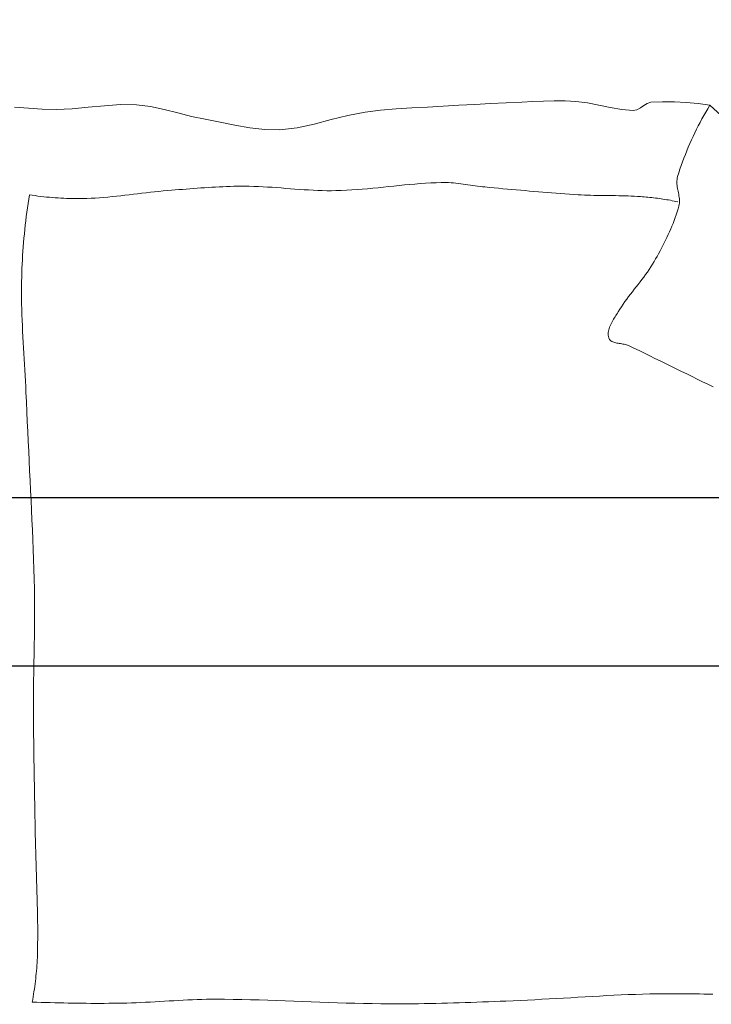
# Model space of a CAD drawing. Units: inches. Extents: x 1484 to 2008, y 1843 to 2590.
# Tile 5 of 21: x 1811 to 1853, y 1981 to 2039. Entities that reach past the tile are written whole.
import ezdxf

# ---------------------------------------------------------------- set-up
doc = ezdxf.new("R2010")
doc.units = ezdxf.units.IN
doc.layers.add('A-ANNO-DIMS', color=2, linetype='Continuous', lineweight=18)
doc.layers.add('A-FURN', color=8, linetype='Continuous', lineweight=18)
doc.styles.get("Standard").update_dxf_attribs({"font": 'arial.ttf'})
doc.dimstyles.new('ISO-25', dxfattribs={"dimtxt": 7, "dimasz": 2.5, "dimexe": 1.25, "dimexo": 0.625, "dimtad": 1, "dimdec": 0, "dimlunit": 3, "dimtxsty": 'Standard', "dimcen": 2.5, "dimadec": 0, "dimazin": 0, "dimtfac": 1, "dimtdec": 0, "dimtmove": 0, "dimatfit": 3, "dimfxl": 1, "dimarcsym": 0})

# ---------------------------------------------------------------- blocks, each defined once
blk = doc.blocks.new('BED-DOUBLE')
for p, q in [((1.063, 49.042), (0.265, 48.148)), ((0.265, 48.148), (0.164, 47.454)), ((0.265, 48.148), (0.464, 48.028)), ((0.464, 48.028), (0.665, 47.91)), ((0.665, 47.91), (0.867, 47.795)), ((16.669, 47.725), (16.821, 48.04)), ((16.821, 48.04), (16.973, 48.355)), ((53.003, 47.799), (53.009, 48.067)), ((53.009, 48.067), (53.016, 48.334)), ((0.164, 47.454), (0.095, 46.755)), ((0.867, 47.795), (1.07, 47.682)), ((1.07, 47.682), (1.275, 47.572)), ((1.275, 47.572), (1.482, 47.465)), ((1.482, 47.465), (1.69, 47.36)), ((1.69, 47.36), (1.899, 47.258)), ((16.362, 47.096), (16.516, 47.41)), ((16.516, 47.41), (16.669, 47.725)), ((52.992, 47.265), (52.997, 47.532)), ((52.997, 47.532), (53.003, 47.799)), ((0.095, 46.755), (0.059, 46.053)), ((1.899, 47.258), (2.11, 47.158)), ((2.11, 47.158), (2.322, 47.061)), ((2.322, 47.061), (2.535, 46.966)), ((2.535, 46.966), (2.749, 46.875)), ((2.749, 46.875), (2.964, 46.786)), ((2.964, 46.786), (3.18, 46.699)), ((16.053, 46.467), (16.208, 46.781)), ((16.208, 46.781), (16.362, 47.096)), ((52.983, 46.731), (52.987, 46.998)), ((52.987, 46.998), (52.992, 47.265)), ((3.18, 46.699), (3.398, 46.616)), ((3.398, 46.616), (3.616, 46.535)), ((3.616, 46.535), (3.835, 46.457)), ((3.835, 46.457), (4.055, 46.382)), ((4.055, 46.382), (4.276, 46.31)), ((4.276, 46.31), (4.498, 46.24)), ((4.498, 46.24), (4.581, 46.219)), ((4.581, 46.219), (4.666, 46.205)), ((4.666, 46.205), (4.752, 46.198)), ((4.752, 46.198), (4.839, 46.197)), ((4.839, 46.197), (4.926, 46.202)), ((4.926, 46.202), (5.014, 46.211)), ((5.014, 46.211), (5.102, 46.223)), ((5.102, 46.223), (5.191, 46.238)), ((5.191, 46.238), (5.279, 46.254)), ((5.279, 46.254), (5.368, 46.272)), ((5.368, 46.272), (5.457, 46.29)), ((5.457, 46.29), (5.546, 46.307)), ((5.546, 46.307), (5.635, 46.322)), ((5.635, 46.322), (5.723, 46.335)), ((5.723, 46.335), (5.811, 46.345)), ((5.811, 46.345), (5.899, 46.351)), ((5.899, 46.351), (5.986, 46.352)), ((5.989, 46.252), (5.966, 46.142)), ((5.986, 46.352), (6.072, 46.347)), ((6.072, 46.347), (6.158, 46.335)), ((6.158, 46.335), (6.242, 46.316)), ((6.242, 46.316), (6.416, 46.266)), ((6.416, 46.266), (6.588, 46.213)), ((6.588, 46.213), (6.76, 46.157)), ((6.76, 46.157), (6.931, 46.097)), ((15.898, 46.154), (16.053, 46.467)), ((52.978, 45.93), (52.979, 46.197)), ((52.979, 46.197), (52.981, 46.464)), ((52.981, 46.464), (52.983, 46.731)), ((0.059, 46.053), (0.056, 45.35)), ((5.864, 45.592), (5.846, 45.481)), ((5.883, 45.702), (5.864, 45.592)), ((5.903, 45.812), (5.883, 45.702)), ((5.923, 45.923), (5.903, 45.812)), ((5.944, 46.032), (5.923, 45.923)), ((5.966, 46.142), (5.944, 46.032)), ((6.931, 46.097), (7.1, 46.035)), ((7.1, 46.035), (7.269, 45.97)), ((7.269, 45.97), (7.437, 45.903)), ((7.437, 45.903), (7.604, 45.833)), ((7.604, 45.833), (7.77, 45.76)), ((7.77, 45.76), (7.935, 45.686)), ((7.935, 45.686), (8.1, 45.609)), ((8.1, 45.609), (8.263, 45.53)), ((15.589, 45.526), (15.743, 45.84)), ((15.743, 45.84), (15.898, 46.154)), ((52.978, 45.663), (52.978, 45.93)), ((52.98, 45.396), (52.978, 45.663)), ((0.056, 45.35), (0.087, 44.65)), ((5.782, 45.038), (5.767, 44.927)), ((5.797, 45.149), (5.782, 45.038)), ((5.812, 45.26), (5.797, 45.149)), ((5.829, 45.371), (5.812, 45.26)), ((5.846, 45.481), (5.829, 45.371)), ((8.263, 45.53), (8.426, 45.45)), ((8.426, 45.45), (8.587, 45.368)), ((8.587, 45.368), (8.748, 45.284)), ((8.748, 45.284), (8.908, 45.199)), ((8.908, 45.199), (9.068, 45.113)), ((9.068, 45.113), (9.226, 45.025)), ((9.226, 45.025), (9.384, 44.936)), ((15.28, 44.897), (15.434, 45.212)), ((15.434, 45.212), (15.589, 45.526)), ((52.983, 45.129), (52.98, 45.396)), ((52.987, 44.862), (52.983, 45.129)), ((0.087, 44.65), (0.148, 44.431)), ((0.148, 44.431), (0.271, 44.228)), ((5.718, 44.482), (5.707, 44.371)), ((5.729, 44.593), (5.718, 44.482)), ((5.741, 44.705), (5.729, 44.593)), ((5.754, 44.816), (5.741, 44.705)), ((5.767, 44.927), (5.754, 44.816)), ((9.384, 44.936), (9.541, 44.847)), ((9.541, 44.847), (9.699, 44.754)), ((9.699, 44.754), (9.854, 44.656)), ((9.854, 44.656), (10.007, 44.555)), ((10.007, 44.555), (10.158, 44.451)), ((10.158, 44.451), (10.307, 44.345)), ((14.974, 44.268), (15.127, 44.583)), ((15.127, 44.583), (15.28, 44.897)), ((52.993, 44.595), (52.987, 44.862)), ((53.005, 44.167), (52.993, 44.595)), ((0.271, 44.228), (0.412, 44.029)), ((0.412, 44.029), (0.528, 43.826)), ((0.528, 43.826), (0.574, 43.607)), ((5.668, 43.852), (5.658, 43.667)), ((5.68, 44.036), (5.668, 43.852)), ((5.688, 44.148), (5.68, 44.036)), ((5.697, 44.259), (5.688, 44.148)), ((5.707, 44.371), (5.697, 44.259)), ((10.307, 44.345), (10.455, 44.236)), ((10.455, 44.236), (10.602, 44.125)), ((10.602, 44.125), (10.748, 44.013)), ((10.748, 44.013), (10.893, 43.9)), ((10.893, 43.9), (11.037, 43.786)), ((14.671, 43.637), (14.822, 43.953)), ((14.822, 43.953), (14.974, 44.268)), ((53.02, 43.74), (53.005, 44.167)), ((0.574, 43.607), (0.52, 42.921)), ((5.643, 43.298), (5.637, 43.113)), ((5.65, 43.483), (5.643, 43.298)), ((5.658, 43.667), (5.65, 43.483)), ((11.037, 43.786), (11.182, 43.672)), ((11.182, 43.672), (11.327, 43.559)), ((11.327, 43.559), (11.472, 43.446)), ((11.472, 43.446), (11.619, 43.334)), ((11.619, 43.334), (11.766, 43.224)), ((14.476, 43.199), (14.497, 43.262)), ((14.497, 43.262), (14.522, 43.32)), ((14.522, 43.32), (14.671, 43.637)), ((53.036, 43.313), (53.02, 43.74)), ((53.055, 42.886), (53.036, 43.313)), ((0.52, 42.921), (0.401, 42.241)), ((5.629, 42.744), (5.626, 42.559)), ((5.633, 42.929), (5.629, 42.744)), ((5.637, 43.113), (5.633, 42.929)), ((11.766, 43.224), (11.914, 43.116)), ((11.914, 43.116), (12.064, 43.01)), ((12.064, 43.01), (12.216, 42.907)), ((12.216, 42.907), (12.37, 42.807)), ((12.37, 42.807), (12.526, 42.712)), ((12.526, 42.712), (12.597, 42.669)), ((12.597, 42.669), (12.668, 42.624)), ((14.372, 42.642), (14.385, 42.711)), ((14.385, 42.711), (14.396, 42.782)), ((14.396, 42.782), (14.407, 42.853)), ((14.407, 42.853), (14.418, 42.925)), ((14.418, 42.925), (14.43, 42.996)), ((14.43, 42.996), (14.443, 43.066)), ((14.443, 43.066), (14.459, 43.134)), ((14.459, 43.134), (14.476, 43.199)), ((53.075, 42.458), (53.055, 42.886)), ((0.401, 42.241), (0.255, 41.563)), ((5.621, 42.189), (5.619, 42.005)), ((5.624, 42.374), (5.621, 42.189)), ((5.626, 42.559), (5.624, 42.374)), ((12.668, 42.624), (12.741, 42.578)), ((12.741, 42.578), (12.814, 42.532)), ((12.814, 42.532), (12.889, 42.485)), ((12.889, 42.485), (12.964, 42.439)), ((12.964, 42.439), (13.04, 42.394)), ((13.04, 42.394), (13.116, 42.35)), ((13.116, 42.35), (13.194, 42.309)), ((13.194, 42.309), (13.271, 42.27)), ((13.271, 42.27), (13.349, 42.234)), ((13.349, 42.234), (13.427, 42.203)), ((13.427, 42.203), (13.506, 42.176)), ((13.506, 42.176), (13.585, 42.153)), ((13.585, 42.153), (13.663, 42.137)), ((13.663, 42.137), (13.742, 42.126)), ((13.742, 42.126), (13.821, 42.122)), ((13.821, 42.122), (13.899, 42.125)), ((13.899, 42.125), (13.978, 42.136)), ((13.978, 42.136), (14.056, 42.155)), ((14.056, 42.155), (14.112, 42.178)), ((14.112, 42.178), (14.161, 42.208)), ((14.161, 42.208), (14.204, 42.244)), ((14.204, 42.244), (14.241, 42.287)), ((14.241, 42.287), (14.272, 42.336)), ((14.272, 42.336), (14.299, 42.389)), ((14.299, 42.389), (14.322, 42.447)), ((14.322, 42.447), (14.341, 42.509)), ((14.341, 42.509), (14.358, 42.574)), ((14.358, 42.574), (14.372, 42.642)), ((53.096, 42.031), (53.075, 42.458)), ((0.255, 41.563), (0.119, 40.884)), ((5.615, 41.635), (5.612, 41.45)), ((5.617, 41.82), (5.615, 41.635)), ((5.619, 42.005), (5.617, 41.82)), ((53.119, 41.604), (53.096, 42.031)), ((53.142, 41.177), (53.119, 41.604)), ((5.604, 41.081), (5.598, 40.896)), ((5.608, 41.265), (5.604, 41.081)), ((5.612, 41.45), (5.608, 41.265)), ((53.166, 40.75), (53.142, 41.177)), ((0.119, 40.884), (0.031, 40.199)), ((5.572, 40.342), (5.556, 40.079)), ((5.582, 40.527), (5.572, 40.342)), ((5.591, 40.711), (5.582, 40.527)), ((5.598, 40.896), (5.591, 40.711)), ((53.191, 40.323), (53.166, 40.75)), ((53.216, 39.896), (53.191, 40.323)), ((0.031, 40.199), (0.001, 39.561)), ((5.539, 39.816), (5.52, 39.554)), ((5.556, 40.079), (5.539, 39.816)), ((53.241, 39.469), (53.216, 39.896)), ((0.001, 39.561), (0, 38.922)), ((5.502, 39.291), (5.482, 39.028)), ((5.52, 39.554), (5.502, 39.291)), ((53.266, 39.043), (53.241, 39.469)), ((0, 38.922), (0.02, 38.282)), ((5.462, 38.766), (5.441, 38.503)), ((5.482, 39.028), (5.462, 38.766)), ((53.29, 38.616), (53.266, 39.043)), ((53.314, 38.189), (53.29, 38.616)), ((0.02, 38.282), (0.048, 37.643)), ((5.397, 37.978), (5.375, 37.715)), ((5.419, 38.24), (5.397, 37.978)), ((5.441, 38.503), (5.419, 38.24)), ((53.337, 37.761), (53.314, 38.189)), ((0.048, 37.643), (0.075, 37.003)), ((5.352, 37.453), (5.329, 37.191)), ((5.375, 37.715), (5.352, 37.453)), ((53.359, 37.334), (53.337, 37.761)), ((0.075, 37.003), (0.114, 36.068)), ((5.306, 36.928), (5.282, 36.666)), ((5.329, 37.191), (5.306, 36.928)), ((53.379, 36.907), (53.359, 37.334)), ((53.398, 36.48), (53.379, 36.907)), ((5.258, 36.403), (5.234, 36.141)), ((5.282, 36.666), (5.258, 36.403)), ((53.415, 36.053), (53.398, 36.48)), ((0.114, 36.068), (0.158, 35.133)), ((5.211, 35.879), (5.187, 35.616)), ((5.234, 36.141), (5.211, 35.879)), ((53.429, 35.707), (53.415, 36.053)), ((53.442, 35.361), (53.429, 35.707)), ((0.158, 35.133), (0.209, 34.198)), ((5.14, 35.091), (5.126, 34.948)), ((5.163, 35.354), (5.14, 35.091)), ((5.187, 35.616), (5.163, 35.354)), ((53.455, 35.016), (53.442, 35.361)), ((5.075, 34.517), (5.055, 34.373)), ((5.093, 34.66), (5.075, 34.517)), ((5.11, 34.804), (5.093, 34.66)), ((5.126, 34.948), (5.11, 34.804)), ((53.468, 34.67), (53.455, 35.016)), ((53.481, 34.324), (53.468, 34.67)), ((0.209, 34.198), (0.263, 33.264)), ((4.994, 33.943), (4.974, 33.799)), ((5.015, 34.086), (4.994, 33.943)), ((5.035, 34.23), (5.015, 34.086)), ((5.055, 34.373), (5.035, 34.23)), ((53.493, 33.978), (53.481, 34.324)), ((53.506, 33.632), (53.493, 33.978)), ((4.917, 33.369), (4.9, 33.225)), ((4.935, 33.512), (4.917, 33.369)), ((4.954, 33.656), (4.935, 33.512)), ((4.974, 33.799), (4.954, 33.656)), ((53.517, 33.287), (53.506, 33.632)), ((0.263, 33.264), (0.321, 32.329)), ((4.862, 32.794), (4.854, 32.65)), ((4.872, 32.938), (4.862, 32.794)), ((4.885, 33.081), (4.872, 32.938)), ((4.9, 33.225), (4.885, 33.081)), ((53.528, 32.941), (53.517, 33.287)), ((53.538, 32.595), (53.528, 32.941)), ((0.321, 32.329), (0.373, 31.4)), ((4.848, 32.506), (4.846, 32.361)), ((4.846, 32.361), (4.847, 32.217)), ((4.847, 32.217), (4.856, 31.904)), ((4.854, 32.65), (4.848, 32.506)), ((53.548, 32.249), (53.538, 32.595)), ((53.556, 31.903), (53.548, 32.249)), ((4.856, 31.904), (4.87, 31.591)), ((4.87, 31.591), (4.888, 31.278)), ((53.564, 31.557), (53.556, 31.903)), ((53.571, 31.211), (53.564, 31.557)), ((0.373, 31.4), (0.421, 30.47)), ((4.888, 31.278), (4.91, 30.965)), ((4.91, 30.965), (4.935, 30.653)), ((53.576, 30.865), (53.571, 31.211)), ((0.421, 30.47), (0.477, 29.541)), ((4.935, 30.653), (4.963, 30.341)), ((53.58, 30.52), (53.576, 30.865)), ((53.583, 30.174), (53.58, 30.52)), ((4.963, 30.341), (4.993, 30.028)), ((4.993, 30.028), (5.024, 29.716)), ((53.585, 29.828), (53.583, 30.174)), ((53.585, 29.482), (53.585, 29.828)), ((0.477, 29.541), (0.554, 28.614)), ((5.024, 29.716), (5.057, 29.404)), ((5.057, 29.404), (5.09, 29.092)), ((53.584, 29.136), (53.585, 29.482)), ((5.09, 29.092), (5.123, 28.78)), ((5.123, 28.78), (5.155, 28.468)), ((53.579, 28.621), (53.584, 29.136)), ((0.554, 28.614), (0.665, 27.691)), ((5.155, 28.468), (5.186, 28.156)), ((5.186, 28.156), (5.216, 27.843)), ((53.561, 27.592), (53.571, 28.107)), ((53.571, 28.107), (53.579, 28.621)), ((0.665, 27.691), (0.86, 26.677)), ((5.216, 27.843), (5.243, 27.531)), ((5.243, 27.531), (5.268, 27.219)), ((53.548, 27.078), (53.561, 27.592)), ((5.268, 27.219), (5.289, 26.906)), ((5.289, 26.906), (5.307, 26.593)), ((53.533, 26.563), (53.548, 27.078)), ((0.86, 26.677), (1.116, 25.673)), ((5.307, 26.593), (5.32, 26.28)), ((53.516, 26.049), (53.533, 26.563)), ((5.32, 26.28), (5.329, 25.967)), ((5.329, 25.967), (5.332, 25.696)), ((53.499, 25.534), (53.516, 26.049)), ((1.116, 25.673), (1.379, 24.67)), ((5.324, 25.155), (5.315, 24.884)), ((5.33, 25.425), (5.324, 25.155)), ((5.332, 25.696), (5.33, 25.425)), ((53.48, 25.02), (53.499, 25.534)), ((1.379, 24.67), (1.595, 23.662)), ((5.303, 24.614), (5.288, 24.343)), ((5.315, 24.884), (5.303, 24.614)), ((53.46, 24.505), (53.48, 25.02)), ((5.271, 24.073), (5.252, 23.802)), ((5.288, 24.343), (5.271, 24.073)), ((53.421, 23.477), (53.441, 23.991)), ((53.441, 23.991), (53.46, 24.505)), ((1.595, 23.662), (1.71, 22.641)), ((5.232, 23.532), (5.212, 23.261)), ((5.252, 23.802), (5.232, 23.532)), ((53.402, 22.962), (53.421, 23.477)), ((5.191, 22.991), (5.17, 22.72)), ((5.212, 23.261), (5.191, 22.991)), ((53.384, 22.448), (53.402, 22.962)), ((1.71, 22.641), (1.697, 21.749)), ((5.15, 22.45), (5.131, 22.179)), ((5.17, 22.72), (5.15, 22.45)), ((53.367, 21.933), (53.384, 22.448)), ((1.697, 21.749), (1.596, 20.86)), ((5.098, 21.638), (5.085, 21.368)), ((5.113, 21.909), (5.098, 21.638)), ((5.131, 22.179), (5.113, 21.909)), ((53.351, 21.419), (53.367, 21.933)), ((5.075, 21.097), (5.068, 20.826)), ((5.085, 21.368), (5.075, 21.097)), ((53.337, 20.905), (53.351, 21.419)), ((1.596, 20.86), (1.44, 19.975)), ((5.068, 20.826), (5.065, 20.555)), ((5.065, 20.555), (5.066, 20.338)), ((53.326, 20.39), (53.337, 20.905)), ((1.44, 19.975), (1.262, 19.091)), ((5.066, 20.338), (5.068, 20.12)), ((5.068, 20.12), (5.072, 19.903)), ((5.072, 19.903), (5.078, 19.685)), ((53.31, 19.361), (53.317, 19.876)), ((53.317, 19.876), (53.326, 20.39)), ((5.078, 19.685), (5.085, 19.468)), ((5.085, 19.468), (5.094, 19.251)), ((53.307, 18.846), (53.31, 19.361)), ((1.262, 19.091), (1.093, 18.209)), ((5.094, 19.251), (5.104, 19.033)), ((5.104, 19.033), (5.115, 18.816)), ((5.115, 18.816), (5.127, 18.599)), ((53.308, 18.568), (53.307, 18.846)), ((1.093, 18.209), (0.922, 17.393)), ((5.127, 18.599), (5.141, 18.382)), ((5.141, 18.382), (5.155, 18.164)), ((5.155, 18.164), (5.17, 17.947)), ((53.312, 18.29), (53.308, 18.568)), ((53.318, 18.011), (53.312, 18.29)), ((5.17, 17.947), (5.186, 17.73)), ((5.186, 17.73), (5.202, 17.513)), ((53.327, 17.733), (53.318, 18.011)), ((53.338, 17.455), (53.327, 17.733)), ((0.922, 17.393), (0.715, 16.583)), ((5.202, 17.513), (5.218, 17.296)), ((5.218, 17.296), (5.235, 17.079)), ((5.235, 17.079), (5.252, 16.862)), ((53.35, 17.177), (53.338, 17.455)), ((53.364, 16.899), (53.35, 17.177)), ((0.715, 16.583), (0.509, 15.773)), ((5.252, 16.862), (5.269, 16.645)), ((5.269, 16.645), (5.286, 16.428)), ((5.286, 16.428), (5.303, 16.211)), ((53.379, 16.62), (53.364, 16.899)), ((53.395, 16.342), (53.379, 16.62)), ((5.303, 16.211), (5.324, 15.959)), ((5.324, 15.959), (5.346, 15.707)), ((53.412, 16.064), (53.395, 16.342)), ((53.429, 15.786), (53.412, 16.064)), ((53.445, 15.508), (53.429, 15.786)), ((0.509, 15.773), (0.338, 14.959)), ((5.346, 15.707), (5.371, 15.456)), ((5.371, 15.456), (5.398, 15.204)), ((5.398, 15.204), (5.426, 14.953)), ((53.462, 15.23), (53.445, 15.508)), ((53.477, 14.952), (53.462, 15.23)), ((0.338, 14.959), (0.237, 14.135)), ((5.426, 14.953), (5.454, 14.702)), ((5.454, 14.702), (5.484, 14.451)), ((53.492, 14.674), (53.477, 14.952)), ((53.506, 14.395), (53.492, 14.674)), ((0.237, 14.135), (0.225, 13.181)), ((5.484, 14.451), (5.514, 14.199)), ((5.514, 14.199), (5.544, 13.948)), ((53.518, 14.117), (53.506, 14.395)), ((53.528, 13.839), (53.518, 14.117)), ((5.544, 13.948), (5.574, 13.697)), ((5.574, 13.697), (5.603, 13.446)), ((5.603, 13.446), (5.631, 13.195)), ((53.536, 13.561), (53.528, 13.839)), ((53.542, 13.282), (53.536, 13.561)), ((0.225, 13.181), (0.286, 12.227)), ((5.631, 13.195), (5.658, 12.943)), ((5.658, 12.943), (5.684, 12.692)), ((53.545, 13.015), (53.542, 13.282)), ((53.548, 12.748), (53.545, 13.015)), ((5.684, 12.692), (5.707, 12.44)), ((5.707, 12.44), (5.729, 12.189)), ((53.55, 12.481), (53.548, 12.748)), ((53.552, 12.214), (53.55, 12.481)), ((0.286, 12.227), (0.381, 11.273)), ((5.729, 12.189), (5.748, 11.937)), ((5.748, 11.937), (5.765, 11.685)), ((53.553, 11.947), (53.552, 12.214)), ((53.553, 11.68), (53.553, 11.947)), ((0.381, 11.273), (0.472, 10.318)), ((5.765, 11.685), (5.778, 11.433)), ((5.778, 11.433), (5.788, 11.18)), ((5.788, 11.18), (5.793, 11.01)), ((53.548, 10.878), (53.55, 11.146)), ((53.55, 11.146), (53.552, 11.413)), ((53.552, 11.413), (53.553, 11.68)), ((5.793, 11.01), (5.796, 10.839)), ((5.796, 10.839), (5.797, 10.669)), ((5.797, 10.669), (5.797, 10.498)), ((53.541, 10.344), (53.545, 10.611)), ((53.545, 10.611), (53.548, 10.878)), ((0.472, 10.318), (0.518, 9.363)), ((5.786, 9.987), (5.78, 9.816)), ((5.792, 10.157), (5.786, 9.987)), ((5.795, 10.328), (5.792, 10.157)), ((5.797, 10.498), (5.795, 10.328)), ((53.531, 9.81), (53.537, 10.077)), ((53.537, 10.077), (53.541, 10.344)), ((0.518, 9.363), (0.498, 8.541)), ((5.762, 9.475), (5.75, 9.305)), ((5.771, 9.646), (5.762, 9.475)), ((5.78, 9.816), (5.771, 9.646)), ((53.519, 9.276), (53.525, 9.543)), ((53.525, 9.543), (53.531, 9.81)), ((5.706, 8.795), (5.688, 8.625)), ((5.722, 8.965), (5.706, 8.795)), ((5.737, 9.135), (5.722, 8.965)), ((5.75, 9.305), (5.737, 9.135)), ((53.503, 8.742), (53.511, 9.009)), ((53.511, 9.009), (53.519, 9.276)), ((0.498, 8.541), (0.441, 7.719)), ((5.647, 8.286), (5.624, 8.117)), ((5.668, 8.456), (5.647, 8.286)), ((5.688, 8.625), (5.668, 8.456)), ((45.254, 8.172), (45.595, 8.182)), ((45.595, 8.182), (45.936, 8.193)), ((45.936, 8.193), (46.277, 8.204)), ((46.277, 8.204), (46.618, 8.215)), ((46.618, 8.215), (46.959, 8.226)), ((46.959, 8.226), (47.3, 8.235)), ((47.3, 8.235), (47.64, 8.244)), ((47.64, 8.244), (47.981, 8.252)), ((47.981, 8.252), (48.322, 8.259)), ((48.322, 8.259), (48.663, 8.264)), ((48.663, 8.264), (49.004, 8.268)), ((49.004, 8.268), (49.345, 8.269)), ((49.345, 8.269), (49.686, 8.269)), ((49.686, 8.269), (50.027, 8.266)), ((50.027, 8.266), (50.368, 8.261)), ((50.368, 8.261), (50.524, 8.258)), ((50.524, 8.258), (50.68, 8.253)), ((50.68, 8.253), (50.836, 8.247)), ((50.836, 8.247), (50.992, 8.239)), ((50.992, 8.239), (51.148, 8.23)), ((51.148, 8.23), (51.304, 8.22)), ((51.304, 8.22), (51.46, 8.209)), ((51.46, 8.209), (51.616, 8.196)), ((51.616, 8.196), (51.772, 8.182)), ((51.772, 8.182), (51.928, 8.166)), ((53.474, 7.941), (53.484, 8.208)), ((53.484, 8.208), (53.494, 8.475)), ((53.494, 8.475), (53.503, 8.742)), ((0.441, 7.719), (0.376, 6.898)), ((5.6, 7.949), (5.574, 7.78)), ((5.574, 7.78), (5.829, 7.739)), ((5.624, 8.117), (5.6, 7.949)), ((5.829, 7.739), (6.085, 7.7)), ((6.085, 7.7), (6.341, 7.663)), ((6.341, 7.663), (6.598, 7.627)), ((6.598, 7.627), (6.855, 7.593)), ((17.279, 7.571), (17.863, 7.596)), ((17.863, 7.596), (18.446, 7.622)), ((18.446, 7.622), (19.03, 7.649)), ((19.03, 7.649), (19.613, 7.676)), ((19.613, 7.676), (20.197, 7.704)), ((20.197, 7.704), (20.78, 7.733)), ((20.78, 7.733), (21.363, 7.761)), ((21.363, 7.761), (21.947, 7.79)), ((21.947, 7.79), (22.53, 7.818)), ((22.53, 7.818), (23.114, 7.846)), ((23.114, 7.846), (23.697, 7.874)), ((23.697, 7.874), (24.281, 7.901)), ((24.281, 7.901), (24.864, 7.927)), ((24.864, 7.927), (25.448, 7.952)), ((25.448, 7.952), (26.031, 7.976)), ((26.031, 7.976), (26.615, 7.998)), ((26.615, 7.998), (27.199, 8.019)), ((27.199, 8.019), (27.783, 8.038)), ((27.783, 8.038), (28.366, 8.055)), ((28.366, 8.055), (28.95, 8.069)), ((28.95, 8.069), (29.311, 8.077)), ((29.311, 8.077), (29.672, 8.081)), ((29.672, 8.081), (30.033, 8.084)), ((30.033, 8.084), (30.394, 8.084)), ((30.394, 8.084), (30.755, 8.083)), ((30.755, 8.083), (31.116, 8.081)), ((31.116, 8.081), (31.477, 8.077)), ((31.477, 8.077), (31.838, 8.072)), ((31.838, 8.072), (32.199, 8.066)), ((32.199, 8.066), (32.56, 8.059)), ((32.56, 8.059), (32.921, 8.053)), ((32.921, 8.053), (33.282, 8.046)), ((33.282, 8.046), (33.643, 8.039)), ((33.643, 8.039), (34.004, 8.033)), ((34.004, 8.033), (34.365, 8.027)), ((34.365, 8.027), (34.725, 8.022)), ((34.725, 8.022), (35.086, 8.018)), ((35.086, 8.018), (35.447, 8.015)), ((35.447, 8.015), (35.808, 8.014)), ((35.808, 8.014), (36.169, 8.014)), ((36.169, 8.014), (36.538, 8.016)), ((36.538, 8.016), (36.907, 8.019)), ((36.907, 8.019), (37.276, 8.022)), ((37.276, 8.022), (37.645, 8.026)), ((37.645, 8.026), (38.014, 8.03)), ((38.014, 8.03), (38.383, 8.035)), ((38.383, 8.035), (38.752, 8.041)), ((38.752, 8.041), (39.121, 8.046)), ((39.121, 8.046), (39.49, 8.053)), ((39.49, 8.053), (39.859, 8.059)), ((39.859, 8.059), (40.228, 8.066)), ((40.228, 8.066), (40.597, 8.073)), ((40.597, 8.073), (40.966, 8.08)), ((40.966, 8.08), (41.335, 8.087)), ((41.335, 8.087), (41.704, 8.094)), ((41.704, 8.094), (42.073, 8.101)), ((42.073, 8.101), (42.442, 8.108)), ((42.442, 8.108), (42.811, 8.115)), ((42.811, 8.115), (43.18, 8.122)), ((43.18, 8.122), (43.549, 8.128)), ((43.549, 8.128), (43.89, 8.135)), ((43.89, 8.135), (44.231, 8.143)), ((44.231, 8.143), (44.572, 8.152)), ((44.572, 8.152), (44.913, 8.161)), ((44.913, 8.161), (45.254, 8.172)), ((51.928, 8.166), (52.083, 8.15)), ((52.083, 8.15), (52.238, 8.132)), ((52.238, 8.132), (52.394, 8.112)), ((52.394, 8.112), (52.549, 8.092)), ((52.549, 8.092), (52.703, 8.07)), ((52.703, 8.07), (52.858, 8.047)), ((52.858, 8.047), (53.012, 8.022)), ((53.012, 8.022), (53.166, 7.997)), ((53.166, 7.997), (53.32, 7.97)), ((53.32, 7.97), (53.474, 7.941)), ((6.855, 7.593), (7.112, 7.562)), ((7.112, 7.562), (7.369, 7.532)), ((7.369, 7.532), (7.626, 7.504)), ((7.626, 7.504), (7.884, 7.477)), ((7.884, 7.477), (8.142, 7.453)), ((8.142, 7.453), (8.4, 7.43)), ((8.4, 7.43), (8.658, 7.41)), ((8.658, 7.41), (8.917, 7.391)), ((8.917, 7.391), (9.175, 7.374)), ((9.175, 7.374), (9.434, 7.359)), ((9.434, 7.359), (9.692, 7.346)), ((9.692, 7.346), (9.951, 7.335)), ((9.951, 7.335), (10.209, 7.326)), ((10.209, 7.326), (10.468, 7.318)), ((10.468, 7.318), (10.727, 7.313)), ((10.727, 7.313), (11.055, 7.309)), ((11.055, 7.309), (11.382, 7.308)), ((11.382, 7.308), (11.71, 7.31)), ((11.71, 7.31), (12.038, 7.316)), ((12.038, 7.316), (12.365, 7.324)), ((12.365, 7.324), (12.693, 7.334)), ((12.693, 7.334), (13.021, 7.346)), ((13.021, 7.346), (13.348, 7.361)), ((13.348, 7.361), (13.676, 7.376)), ((13.676, 7.376), (14.003, 7.393)), ((14.003, 7.393), (14.331, 7.411)), ((14.331, 7.411), (14.659, 7.43)), ((14.659, 7.43), (14.986, 7.449)), ((14.986, 7.449), (15.314, 7.468)), ((15.314, 7.468), (15.641, 7.487)), ((15.641, 7.487), (15.969, 7.506)), ((15.969, 7.506), (16.296, 7.524)), ((16.296, 7.524), (16.624, 7.541)), ((16.624, 7.541), (16.951, 7.557)), ((16.951, 7.557), (17.279, 7.571))]:
    blk.add_line(p, q)
blk = doc.blocks.new('*D9')
at = {"layer": 'A-ANNO-DIMS', "color": 0, "lineweight": -2, "transparency": 16777216}
for p, q in [((1804.291, 1973.808), (1804.291, 1960.431)), ((1889.307, 1973.808), (1889.307, 1960.431)), ((1806.791, 1961.681), (1886.807, 1961.681)), ((1889.307, 1961.681), (2001.132, 1961.681))]:
    blk.add_line(p, q, dxfattribs=at)
at = {"layer": 'A-ANNO-DIMS', "color": 0, "transparency": 16777216}
for points in [[(1806.791, 1962.097), (1806.791, 1961.264), (1804.291, 1961.681)], [(1886.807, 1962.097), (1886.807, 1961.264), (1889.307, 1961.681)]]:
    blk.add_solid(points, dxfattribs=at)
at = {"layer": 'Defpoints', "color": 0, "transparency": 16777216}
for p in [(1804.291, 1974.433), (1889.307, 1974.433), (1889.307, 1961.681)]:
    blk.add_point(p, dxfattribs=at)
at = {"layer": 'A-ANNO-DIMS', "color": 0, "transparency": 16777216, "insert": (1946.47, 1965.927), "char_height": 7, "attachment_point": 5}
blk.add_mtext('DOUBLE BED 7\'-1" TYP.', dxfattribs=at)
blk = doc.blocks.new('*D32')
at = {"layer": 'A-ANNO-DIMS', "color": 0, "lineweight": -2, "transparency": 16777216}
for p, q in [((1961.855, 2010.803), (1961.855, 2038.599)), ((1648.545, 2010.803), (1963.105, 2010.803)), ((1961.855, 2003.303), (1961.855, 2008.303)), ((1648.545, 2000.803), (1963.105, 2000.803))]:
    blk.add_line(p, q, dxfattribs=at)
at = {"layer": 'A-ANNO-DIMS', "color": 0, "transparency": 16777216}
for points in [[(1961.438, 2008.303), (1962.271, 2008.303), (1961.855, 2010.803)], [(1961.438, 2003.303), (1962.271, 2003.303), (1961.855, 2000.803)]]:
    blk.add_solid(points, dxfattribs=at)
at = {"layer": 'Defpoints', "color": 0, "transparency": 16777216}
for p in [(1647.92, 2010.803), (1961.855, 2010.803), (1647.92, 2000.803)]:
    blk.add_point(p, dxfattribs=at)
at = {"layer": 'A-ANNO-DIMS', "color": 0, "transparency": 16777216, "insert": (1957.656, 2025.951), "char_height": 7, "attachment_point": 5, "rotation": 90}
blk.add_mtext('0\'-10"', dxfattribs=at)

msp = doc.modelspace()

# ---------------------------------------------------------------- block references
at = {"layer": 'A-FURN', "rotation": 269.9999999999906}
msp.add_blockref('BED-DOUBLE', (1804.291, 2034.333), dxfattribs=at)

# ---------------------------------------------------------------- dimensions: what is measured, and where the dimension line sits
at = {"layer": 'A-ANNO-DIMS'}
dim = msp.add_linear_dim(base=(1961.855, 2010.803), p1=(1647.92, 2000.803), p2=(1647.92, 2010.803), angle=90, dimstyle='ISO-25', override={"dimdec": 1, "dimlfac": 1, "dimrnd": 0, "dimzin": 1, "dimdsep": 46, "dimlunit": 4, "dimfrac": 2}, dxfattribs=at)
dim.commit()
dim.dimension.update_dxf_attribs({"geometry": '*D32', "text_midpoint": (1957.656, 2025.951)})
dim = msp.add_linear_dim(base=(1889.307, 1961.681), p1=(1804.291, 1974.433), p2=(1889.307, 1974.433), text='DOUBLE BED <> TYP.', dimstyle='ISO-25', override={"dimdec": 1, "dimlfac": 1, "dimrnd": 0, "dimzin": 1, "dimdsep": 46, "dimlunit": 4, "dimfrac": 2}, dxfattribs=at)
dim.commit()
dim.dimension.update_dxf_attribs({"geometry": '*D9', "text_midpoint": (1946.47, 1965.927)})

doc.saveas('drawing.dxf')
